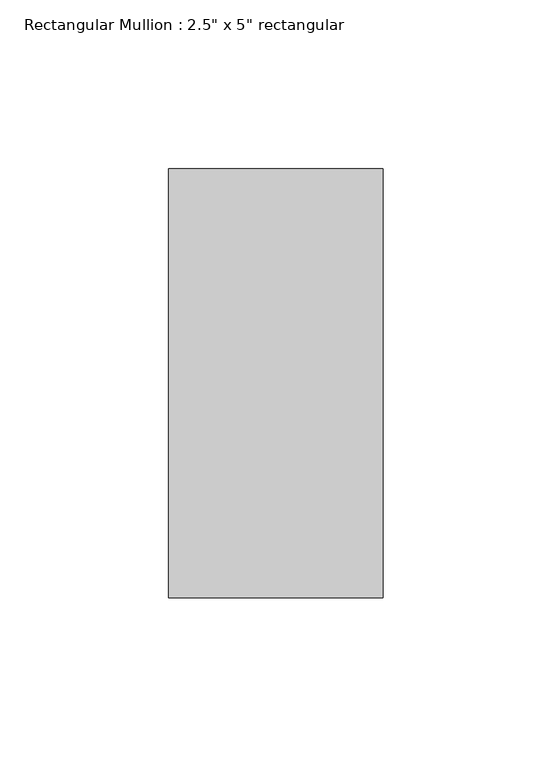
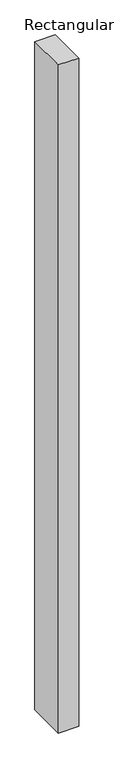
"""IFC4 building model written with IfcOpenShell, lengths in millimetres: member geometry."""

from ifc_helpers import new_model, si_unit, frame, origin, place, context, project, spatial, polyline, outline, extrude, source, transform, mapped, element, save


def member_71d3972c(model_context):
    return source(origin(), model_context, "Body", "SweptSolid", [
        extrude(outline(polyline([(31.75, 63.5), (31.75, -63.5), (-31.75, -63.5), (-31.75, 63.5), (31.75, 63.5)])), frame((0.0, 0.0, -2208.0093941), z_axis=(0.0, 0.0, 1.0), x_axis=(1.0, 0.0, 0.0)), (0.0, 0.0, 1.0), 2208.0093941),
    ])


if __name__ == "__main__":
    model = new_model("IFC4")
    model_context = context("Model", 3, world=origin())
    ifc_project = project(units=[si_unit("LENGTHUNIT", "METRE", prefix="MILLI")], contexts=[model_context])
    site = spatial("IfcSite", under=ifc_project)
    building = spatial("IfcBuilding", under=site)
    placement = place(None, origin())
    member_shape = member_71d3972c(model_context)
    element("IfcMember", 1, ObjectType="Rectangular Mullion : 2.5\" x 5\" rectangular", at=placement, inside=building, context=model_context, shape_type="MappedRepresentation", body=[
        mapped(member_shape, transform((0.0, 0.0, 0.0), x_axis=(1.0, 0.0, 0.0), y_axis=(0.0, 1.0, 0.0), z_axis=(0.0, 0.0, 1.0))),
    ])
    save(model, "model.ifc")

# Revit data of these elements
# Type "Rectangular Mullion : 2.5\" x 5\" rectangular"
#   built-in parameter 1007304 = 0.416667 (stored number, unit not read)
#   built-in parameter 1007301 = 0.104167 (stored number, unit not read)
#   built-in parameter 1007300 = 0.104167 (stored number, unit not read)
